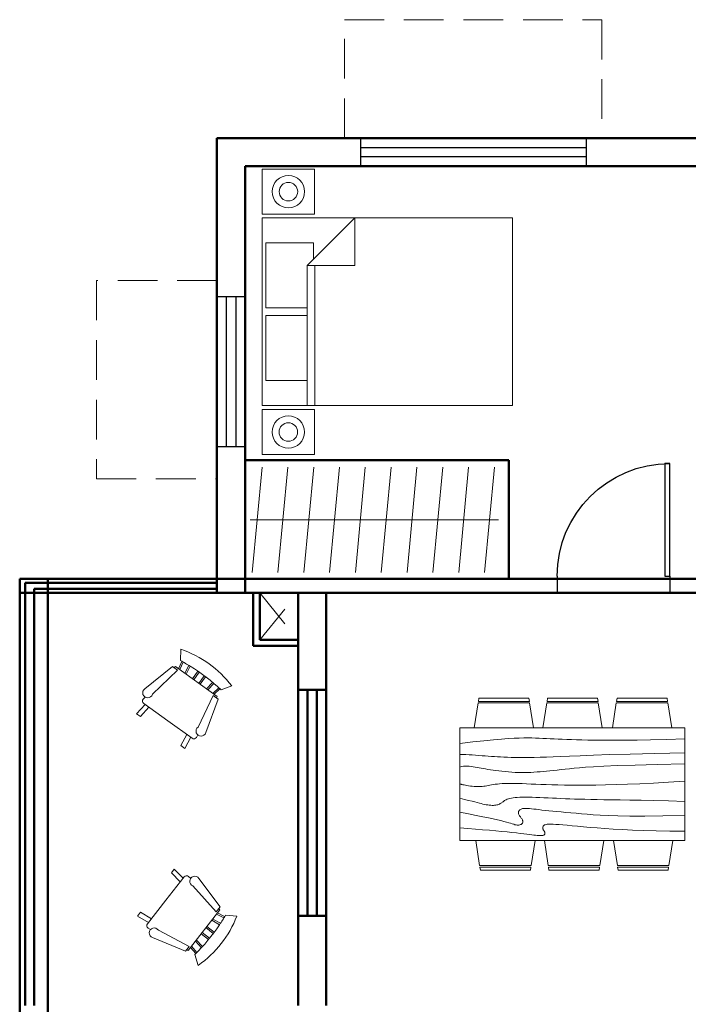
# Model space of a CAD drawing. Units: inches. Extents: x 4795 to 6024, y 2716 to 5025.
# Tile 2 of 19: x 4830 to 5044, y 2917 to 3232. Entities that reach past the tile are written whole.
import ezdxf

# ---------------------------------------------------------------- set-up
doc = ezdxf.new("R2010")
doc.units = ezdxf.units.IN
doc.linetypes.add('DASHED', pattern=[19.05, 12.7, -6.35])
for name, color, linetype, lineweight in [('A-DOOR', 4, 'Continuous', 25), ('A-FURN', 8, 'Continuous', 18), ('A-GLAZ', 4, 'Continuous', 25), ('A-WALL', 7, 'Continuous', 50), ('A-WALL-OVHD', 8, 'DASHED', 18)]:
    doc.layers.add(name, color=color, linetype=linetype, lineweight=lineweight)

# ---------------------------------------------------------------- blocks, each defined once
blk = doc.blocks.new('*U2')
for p, q in [((0, 0), (0, -6)), ((40, 0), (40, -6))]:
    blk.add_line(p, q)
blk.add_lwpolyline([(0, 0), (0, 40), (1.75, 40), (1.75, 0)], close=True)
blk.add_arc((0, 0), 40, 0, 90)
blk = doc.blocks.new('Chair - Rocking')
for p, q in [((-8, -4.5), (-10, -1.5)), ((8, -4.5), (10, -1.5)), ((-7.5, -4.5), (-7, -7)), ((-6.5, -7), (-7.02225, -4.43)), ((-4.5, -7), (-4.96674, -4.19951)), ((-4, -7), (-4.40532, -4.16272)), ((-1.5, -4.05012), (-1.5, -7)), ((-1, -7), (-1, -4.05012)), ((1, -7), (1, -4.04655)), ((1.5, -4.05012), (1.5, -7)), ((4, -7), (4.40187, -4.18694)), ((4.5, -7), (4.96761, -4.19437)), ((6.5, -7), (7, -4.4057)), ((7.5, -4.5), (7, -7)), ((-9, -7.5), (-12, -18.49999)), ((-7, -7.5), (-9, -7.5)), ((-9, -18.49999), (-7, -7.5)), ((-8.23428, -6.99939), (-8.3093, -7.47958)), ((-8.23041, -7), (8.23915, -7)), ((7, -7.5), (9, -7.5)), ((9, -18.49999), (7, -7.5)), ((8.31071, -7.48854), (8.23449, -7.00073)), ((9, -7.5), (12, -18.49999)), ((-10.36644, -20.64523), (-10.5, -21.49999)), ((10.5, -21.49999), (10.3575, -20.58798)), ((-9, -22.49999), (-9.5, -26.49999)), ((0, -22.49999), (-9.5, -22.49999)), ((-8, -26.49999), (-7.5, -22.49999)), ((0, -22.49999), (9.5, -22.49999)), ((8, -26.49999), (7.5, -22.49999)), ((9, -22.49999), (9.5, -26.49999)), ((-9.5, -26.49999), (-8, -26.49999)), ((9.5, -26.49999), (8, -26.49999))]:
    blk.add_line(p, q)
for centre, radius, start, end in [((0, -34.08333), 34.08333, 72.93847, 107.0615), ((0, -68.25004), 64.25, 93.92211, 97.15267), ((0, -68.25004), 64.25, 82.84733, 93.92211), ((-10.5, -18.99999), 1.58114, 161.5651, 18.43495), ((10.5, -18.99999), 1.58114, 161.5651, 18.43495), ((-9.5, -21.49999), 1, 180, 270), ((9.5, -21.49999), 1, 270, 0)]:
    blk.add_arc(centre, radius, start, end)
blk = doc.blocks.new('Bed - Queen')
for p, q in [((0, -80.00003), (0, 0)), ((0, 0), (59.99999, 0)), ((59.99999, 0), (59.99999, -80.00003)), ((7.99999, -1.2), (28.79998, -1.2)), ((7.99999, -14.4), (7.99999, -1.2)), ((28.79998, -1.2), (28.79998, -14.4)), ((31.19999, -1.2), (51.99999, -1.2)), ((31.19999, -14.4), (31.19999, -1.2)), ((51.99999, -1.2), (51.99999, -16.4)), ((0, -14.4), (44.8, -14.4)), ((59.99999, -29.6), (44.8, -14.4)), ((44.8, -14.4), (44.8, -29.6)), ((44.8, -16.8), (0, -16.8)), ((51.99999, -16.4), (46.79936, -16.4)), ((44.8, -29.6), (59.99999, -29.6)), ((59.99999, -80.00003), (0, -80.00003))]:
    blk.add_line(p, q)
blk = doc.blocks.new('WIN-48')
for p, q in [((0, 0), (0, 48)), ((0, 48), (9, 48)), ((3, 0), (3, 48)), ((6, 48), (6, 0)), ((9, 48), (9, 0)), ((9, 0), (0, 0))]:
    blk.add_line(p, q)
blk = doc.blocks.new('WIN-72')
for p, q in [((0, 0), (0, 9)), ((0, 9), (72, 9)), ((72, 9), (72, 0)), ((0, 6), (72, 6)), ((72, 3), (0, 3)), ((72, 0), (0, 0))]:
    blk.add_line(p, q)
blk = doc.blocks.new('CHAIR-DINING')
for p, q in [((8, 17.72), (0, 18.97)), ((8, 17.71), (8, 1.25)), ((9.5, 17.48), (8.5, 17.64)), ((8.5, 1.33), (8.5, 17.64)), ((9.5, 17.48), (9.5, 1.48)), ((0, 0), (8, 1.25)), ((8.5, 1.33), (9.5, 1.48))]:
    blk.add_line(p, q)

msp = doc.modelspace()

# ---------------------------------------------------------------- linework, layer by layer
at = {"layer": 'A-FURN'}
for p, q in [((4904.23, 3055.32), (4907.39, 3088.94)), ((4912.48, 3055.32), (4915.65, 3088.94)), ((4920.74, 3055.32), (4923.9, 3088.94)), ((4928.99, 3055.32), (4932.16, 3088.94)), ((4937.25, 3055.32), (4940.41, 3088.94)), ((4945.5, 3055.32), (4948.67, 3088.94)), ((4953.76, 3055.32), (4956.92, 3088.94)), ((4962.01, 3055.32), (4965.18, 3088.94)), ((4970.26, 3055.32), (4973.43, 3088.94)), ((4978.52, 3055.32), (4981.68, 3088.94)), ((4903.57, 3072.13), (4983.02, 3072.13)), ((5042.59, 3005.57), (4970.59, 3005.57)), ((4970.59, 3005.57), (4970.59, 2969.57)), ((5042.59, 2969.57), (5042.59, 3005.57)), ((4970.59, 2969.57), (5042.59, 2969.57))]:
    msp.add_line(p, q, dxfattribs=at)
for points in [[(4907.45, 3184.32), (4924.18, 3184.32), (4924.18, 3169.91), (4907.45, 3169.91)], [(4907.43, 3107.44), (4924.16, 3107.44), (4924.16, 3093.02), (4907.43, 3093.02)]]:
    msp.add_lwpolyline(points, close=True, dxfattribs=at)
for points in [[(5042.59, 3002.07), (5036.68, 3001.9), (5031.62, 3001.78), (5027.32, 3001.69), (5023.67, 3001.64), (5020.56, 3001.61), (5017.89, 3001.61), (5015.56, 3001.62), (5013.46, 3001.65), (5011.51, 3001.68), (5009.68, 3001.73), (5007.96, 3001.77), (5006.34, 3001.83), (5004.82, 3001.88), (5003.39, 3001.94), (5002.04, 3002), (5000.76, 3002.07), (4999.53, 3002.13), (4998.35, 3002.19), (4997.2, 3002.24), (4996.04, 3002.29), (4994.87, 3002.33), (4993.66, 3002.35), (4992.39, 3002.36), (4991.05, 3002.36), (4989.6, 3002.33), (4987.97, 3002.27), (4986.11, 3002.17), (4983.93, 3002.01), (4981.36, 3001.78), (4978.33, 3001.47), (4974.76, 3001.07), (4970.59, 3000.57)], [(5042.59, 2997.57), (5032.99, 2997.38), (5025.06, 2997.2), (5018.57, 2997.02), (5013.33, 2996.85), (5009.11, 2996.69), (5005.71, 2996.55), (5002.91, 2996.42), (5000.51, 2996.32), (4998.31, 2996.23), (4996.29, 2996.17), (4994.42, 2996.13), (4992.69, 2996.11), (4991.1, 2996.1), (4989.63, 2996.11), (4988.27, 2996.12), (4987.01, 2996.15), (4985.83, 2996.18), (4984.72, 2996.23), (4983.67, 2996.28), (4982.66, 2996.33), (4981.68, 2996.39), (4980.71, 2996.46), (4979.74, 2996.53), (4978.76, 2996.61), (4977.74, 2996.69), (4976.71, 2996.77), (4975.66, 2996.84), (4974.61, 2996.92), (4973.57, 2996.98), (4972.55, 2997.02), (4971.55, 2997.06), (4970.59, 2997.07)], [(5042.59, 2994.07), (5033.77, 2993.88), (5026.67, 2993.69), (5021.06, 2993.51), (5016.7, 2993.33), (5013.36, 2993.15), (5010.83, 2992.98), (5008.85, 2992.81), (5007.21, 2992.65), (5005.72, 2992.5), (5004.32, 2992.35), (5003, 2992.22), (5001.76, 2992.09), (5000.58, 2991.97), (4999.46, 2991.85), (4998.38, 2991.75), (4997.34, 2991.65), (4996.32, 2991.56), (4995.32, 2991.48), (4994.32, 2991.41), (4993.34, 2991.36), (4992.35, 2991.32), (4991.36, 2991.3), (4990.36, 2991.3), (4989.34, 2991.32), (4988.3, 2991.36), (4987.24, 2991.42), (4986.19, 2991.5), (4985.14, 2991.6), (4984.11, 2991.7), (4983.12, 2991.82), (4982.16, 2991.94), (4981.26, 2992.07), (4980.41, 2992.19), (4979.62, 2992.32), (4978.87, 2992.44), (4978.17, 2992.56), (4977.49, 2992.68), (4976.83, 2992.8), (4976.19, 2992.91), (4975.55, 2993.02), (4974.91, 2993.13), (4974.26, 2993.22), (4973.62, 2993.3), (4972.99, 2993.34), (4972.37, 2993.35), (4971.76, 2993.31), (4971.16, 2993.22), (4970.59, 2993.07)], [(5042.59, 2988.57), (5037.38, 2988.23), (5032.61, 2987.95), (5028.24, 2987.73), (5024.25, 2987.56), (5020.59, 2987.44), (5017.24, 2987.35), (5014.17, 2987.3), (5011.34, 2987.27), (5008.72, 2987.27), (5006.3, 2987.28), (5004.06, 2987.3), (5001.97, 2987.34), (5000.04, 2987.39), (4998.23, 2987.44), (4996.53, 2987.5), (4994.92, 2987.57), (4993.4, 2987.63), (4991.96, 2987.69), (4990.59, 2987.74), (4989.31, 2987.78), (4988.11, 2987.82), (4986.99, 2987.84), (4985.96, 2987.84), (4985.01, 2987.82), (4984.14, 2987.77), (4983.35, 2987.71), (4982.63, 2987.63), (4981.97, 2987.55), (4981.37, 2987.45), (4980.8, 2987.35), (4980.27, 2987.25), (4979.76, 2987.15), (4979.26, 2987.06), (4978.78, 2986.98), (4978.3, 2986.91), (4977.82, 2986.86), (4977.33, 2986.82), (4976.83, 2986.8), (4976.3, 2986.8), (4975.76, 2986.82), (4975.18, 2986.86), (4974.59, 2986.92), (4974, 2986.99), (4973.43, 2987.08), (4972.89, 2987.16), (4972.4, 2987.25), (4971.97, 2987.33), (4971.63, 2987.4), (4971.38, 2987.45), (4971.2, 2987.5), (4971.09, 2987.53), (4971, 2987.55), (4970.93, 2987.56), (4970.85, 2987.56), (4970.75, 2987.57), (4970.59, 2987.57)], [(5042.59, 2982.07), (5037.31, 2982.23), (5032.66, 2982.36), (5028.58, 2982.45), (5025.02, 2982.51), (5021.89, 2982.56), (5019.14, 2982.59), (5016.7, 2982.62), (5014.51, 2982.65), (5012.5, 2982.68), (5010.65, 2982.73), (5008.93, 2982.77), (5007.33, 2982.83), (5005.82, 2982.88), (5004.37, 2982.94), (5002.97, 2983), (5001.59, 2983.07), (5000.22, 2983.13), (4998.85, 2983.19), (4997.52, 2983.24), (4996.21, 2983.3), (4994.96, 2983.34), (4993.76, 2983.37), (4992.63, 2983.39), (4991.59, 2983.4), (4990.64, 2983.39), (4989.77, 2983.37), (4988.99, 2983.33), (4988.29, 2983.27), (4987.66, 2983.2), (4987.1, 2983.12), (4986.61, 2983.02), (4986.17, 2982.9), (4985.79, 2982.77), (4985.46, 2982.62), (4985.16, 2982.47), (4984.9, 2982.31), (4984.66, 2982.14), (4984.44, 2981.97), (4984.22, 2981.81), (4984.01, 2981.65), (4983.78, 2981.5), (4983.55, 2981.36), (4983.3, 2981.22), (4983.04, 2981.11), (4982.75, 2981.01), (4982.45, 2980.92), (4982.12, 2980.86), (4981.76, 2980.82), (4981.37, 2980.8), (4980.95, 2980.8), (4980.5, 2980.82), (4980.04, 2980.87), (4979.55, 2980.93), (4979.05, 2981.02), (4978.53, 2981.12), (4978.01, 2981.23), (4977.47, 2981.37), (4976.88, 2981.52), (4976.22, 2981.7), (4975.45, 2981.9), (4974.54, 2982.13), (4973.45, 2982.4), (4972.14, 2982.71), (4970.59, 2983.07)], [(5042.59, 2977.57), (5035.57, 2977.42), (5029.76, 2977.36), (5025.01, 2977.37), (5021.16, 2977.43), (5018.03, 2977.54), (5015.47, 2977.67), (5013.3, 2977.82), (5011.38, 2977.98), (5009.56, 2978.14), (5007.81, 2978.28), (5006.15, 2978.42), (5004.56, 2978.56), (5003.06, 2978.69), (5001.65, 2978.81), (5000.32, 2978.94), (4999.09, 2979.07), (4997.95, 2979.19), (4996.9, 2979.31), (4995.94, 2979.43), (4995.06, 2979.53), (4994.26, 2979.63), (4993.55, 2979.71), (4992.91, 2979.77), (4992.34, 2979.82), (4991.84, 2979.84), (4991.41, 2979.83), (4991.04, 2979.81), (4990.71, 2979.76), (4990.44, 2979.7), (4990.21, 2979.62), (4990.01, 2979.52), (4989.84, 2979.4), (4989.69, 2979.27), (4989.58, 2979.12), (4989.48, 2978.96), (4989.41, 2978.8), (4989.37, 2978.62), (4989.36, 2978.44), (4989.38, 2978.25), (4989.42, 2978.07), (4989.5, 2977.88), (4989.6, 2977.69), (4989.72, 2977.5), (4989.86, 2977.32), (4990, 2977.13), (4990.15, 2976.94), (4990.29, 2976.75), (4990.42, 2976.57), (4990.54, 2976.38), (4990.64, 2976.19), (4990.71, 2976.01), (4990.77, 2975.83), (4990.79, 2975.65), (4990.79, 2975.48), (4990.75, 2975.31), (4990.67, 2975.15), (4990.56, 2975), (4990.41, 2974.86), (4990.23, 2974.73), (4990.02, 2974.63), (4989.78, 2974.55), (4989.51, 2974.49), (4989.23, 2974.47), (4988.92, 2974.48), (4988.6, 2974.53), (4988.25, 2974.62), (4987.85, 2974.74), (4987.4, 2974.88), (4986.87, 2975.06), (4986.26, 2975.25), (4985.54, 2975.46), (4984.71, 2975.69), (4983.75, 2975.93), (4982.63, 2976.19), (4981.31, 2976.48), (4979.76, 2976.8), (4977.95, 2977.16), (4975.84, 2977.57), (4973.4, 2978.04), (4970.59, 2978.57)], [(5042.59, 2972.57), (5037.77, 2972.59), (5033.4, 2972.65), (5029.44, 2972.75), (5025.87, 2972.88), (5022.63, 2973.03), (5019.69, 2973.2), (5017.01, 2973.38), (5014.55, 2973.57), (5012.28, 2973.75), (5010.19, 2973.94), (5008.28, 2974.11), (5006.55, 2974.27), (5004.99, 2974.42), (5003.61, 2974.55), (5002.39, 2974.66), (5001.34, 2974.73), (5000.45, 2974.78), (4999.71, 2974.8), (4999.1, 2974.79), (4998.61, 2974.75), (4998.22, 2974.7), (4997.92, 2974.62), (4997.68, 2974.52), (4997.51, 2974.4), (4997.37, 2974.27), (4997.27, 2974.12), (4997.2, 2973.97), (4997.16, 2973.81), (4997.15, 2973.64), (4997.17, 2973.47), (4997.2, 2973.31), (4997.26, 2973.15), (4997.33, 2973), (4997.41, 2972.85), (4997.49, 2972.71), (4997.58, 2972.58), (4997.66, 2972.45), (4997.74, 2972.32), (4997.8, 2972.19), (4997.84, 2972.07), (4997.86, 2971.94), (4997.85, 2971.82), (4997.83, 2971.7), (4997.78, 2971.59), (4997.7, 2971.48), (4997.6, 2971.39), (4997.48, 2971.3), (4997.34, 2971.23), (4997.17, 2971.18), (4996.97, 2971.14), (4996.74, 2971.12), (4996.46, 2971.11), (4996.14, 2971.12), (4995.77, 2971.14), (4995.34, 2971.18), (4994.84, 2971.23), (4994.27, 2971.3), (4993.62, 2971.39), (4992.87, 2971.49), (4992.02, 2971.6), (4991.05, 2971.72), (4989.95, 2971.85), (4988.7, 2972), (4987.3, 2972.15), (4985.73, 2972.31), (4984, 2972.48), (4982.12, 2972.65), (4980.08, 2972.83), (4977.91, 2973.01), (4975.6, 2973.19), (4973.15, 2973.38), (4970.59, 2973.57)]]:
    msp.add_lwpolyline(points, dxfattribs=at)
for centre, radius in [((4915.82, 3177.12), 5.18), ((4915.82, 3177.12), 2.96), ((4915.79, 3100.23), 5.18), ((4915.79, 3100.23), 2.96)]:
    msp.add_circle(centre, radius, dxfattribs=at)
at = {"layer": 'A-WALL'}
for p, q in [((5286.97, 3194.24), (4892.97, 3194.24)), ((4892.97, 3185.24), (4892.97, 3194.24)), ((4892.97, 3185.24), (4892.97, 3048.74)), ((5286.97, 3185.24), (4901.97, 3185.24)), ((4901.97, 3185.24), (4901.97, 3048.74)), ((4901.97, 3091.21), (4986.25, 3091.21)), ((4986.25, 3091.21), (4986.25, 3053.24)), ((4829.88, 3053.24), (4829.88, 2912.24)), ((4892.97, 3053.24), (4829.88, 3053.24)), ((4838.88, 3053.24), (4838.88, 2912.24)), ((5050.47, 3053.24), (4892.97, 3053.24)), ((4892.97, 3052), (4831.6, 3052)), ((4831.6, 3052), (4831.6, 2916.74)), ((4892.97, 3050.08), (4834.52, 3050.08)), ((4834.52, 3050.08), (4834.52, 2916.74)), ((4892.97, 3048.74), (4829.88, 3048.74)), ((5050.47, 3048.74), (4892.97, 3048.74)), ((4904.55, 3048.74), (4904.55, 3031.86)), ((4906.63, 3048.74), (4906.63, 3033.72)), ((4918.88, 3048.74), (4918.88, 2916.74)), ((4927.88, 3048.74), (4927.88, 2916.74)), ((4906.63, 3033.72), (4918.88, 3033.72)), ((4904.55, 3031.86), (4918.88, 3031.86)), ((4918.88, 3017.81), (4927.88, 3017.81)), ((4921.95, 3017.81), (4921.95, 2945.45)), ((4924.88, 3017.81), (4924.88, 2945.45)), ((4918.88, 2945.45), (4927.88, 2945.45))]:
    msp.add_line(p, q, dxfattribs=at)
at = {"layer": 'A-WALL-OVHD'}
for p, q in [((4933.7, 3194.24), (4933.7, 3232.13)), ((4933.7, 3232.13), (5016.09, 3232.13)), ((5016.09, 3232.13), (5016.09, 3194.24)), ((4892.97, 3148.67), (4854.42, 3148.67)), ((4854.42, 3148.67), (4854.42, 3085.24)), ((4854.42, 3085.24), (4892.97, 3085.24)), ((4906.63, 3048.74), (4918.88, 3033.72)), ((4906.63, 3033.72), (4918.88, 3048.74))]:
    msp.add_line(p, q, dxfattribs=at)

# ---------------------------------------------------------------- block references
at = {"layer": 'A-DOOR', "xscale": -0.9, "yscale": 0.9, "zscale": 0.9}
msp.add_blockref('*U2', (5037.74, 3054.14), dxfattribs=at)
at = {"layer": 'A-FURN'}
for name, p, rotation in [('Bed - Queen', (4907.43, 3108.73), 90), ('Chair - Rocking', (4890.43, 3026.1), 324.2775344515209), ('CHAIR-DINING', (4994.19, 3005.57), 90.00567182442212), ('CHAIR-DINING', (5016.17, 3005.57), 90.00567182441947), ('CHAIR-DINING', (5038.39, 3005.57), 90.0056718244202), ('CHAIR-DINING', (4975.72, 2969.57), 270.0000000000044), ('CHAIR-DINING', (4997.66, 2969.57), 270.0000000000017), ('CHAIR-DINING', (5019.76, 2969.57), 270.0000000000017), ('Chair - Rocking', (4894.34, 2936.58), 232.0049313276433)]:
    msp.add_blockref(name, p, dxfattribs=dict(at, rotation=rotation))
at = {"layer": 'A-GLAZ', "rotation": 180}
msp.add_blockref('WIN-72', (5011.01, 3194.24), dxfattribs=at)
at = {"layer": 'A-GLAZ'}
msp.add_blockref('WIN-48', (4892.97, 3095.54), dxfattribs=at)

doc.saveas('drawing.dxf')
